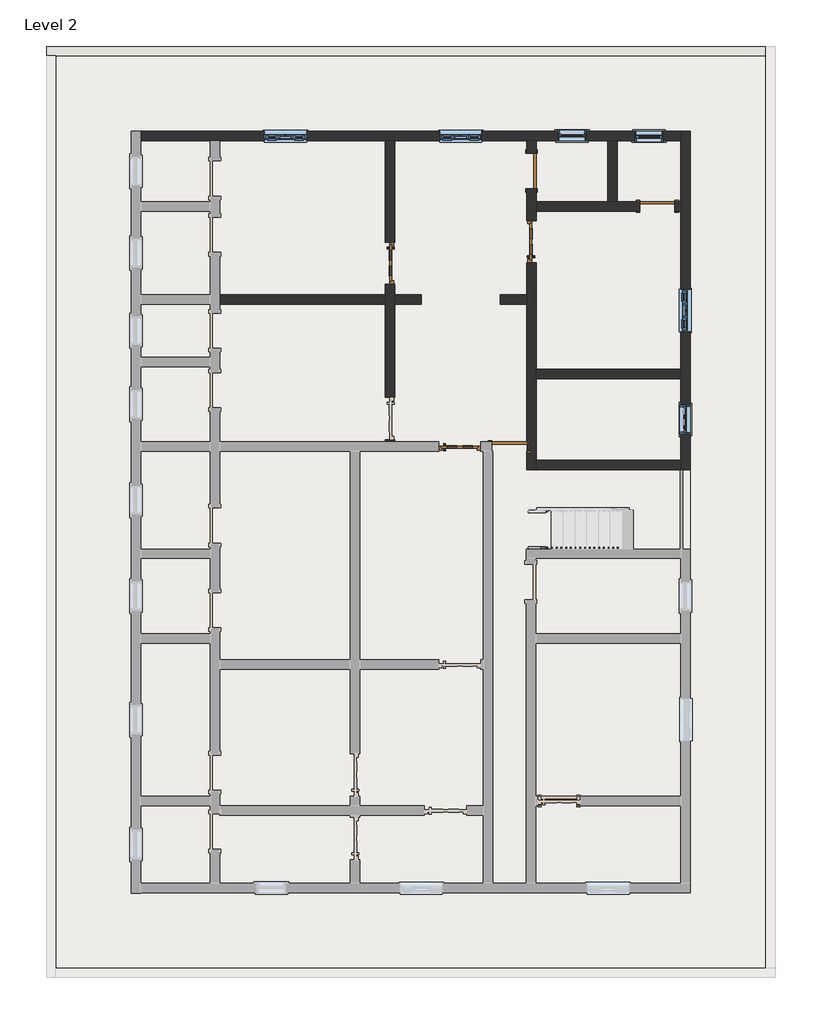
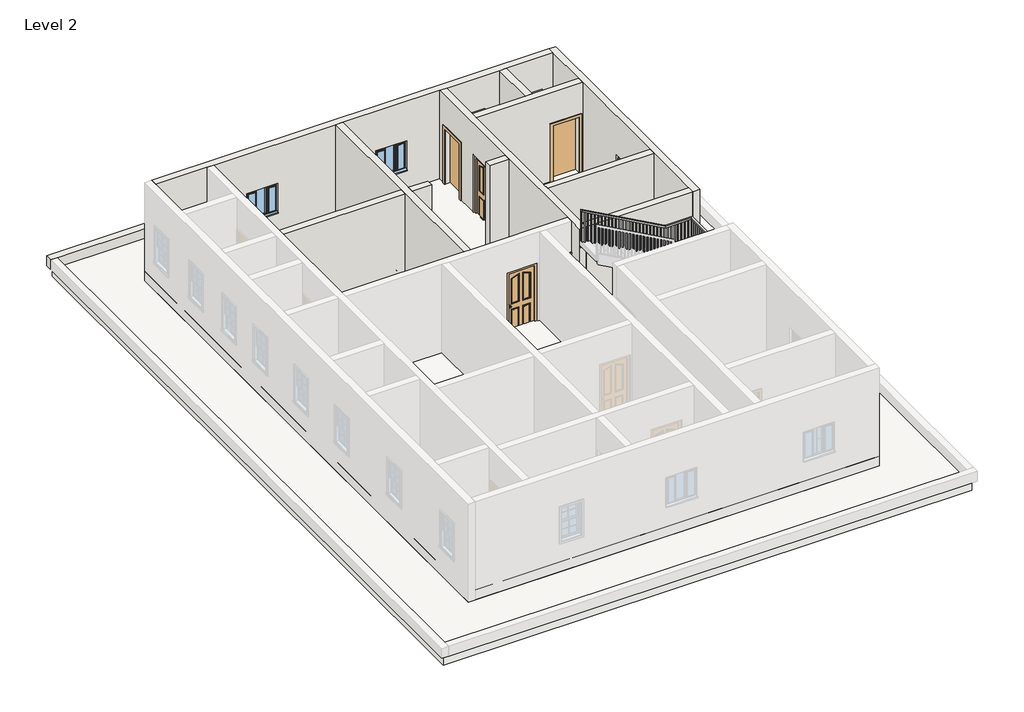
# One storey, part 2 of 3: 11 walls, 6 doors, 6 windows, 2 slabs, 1 railing, 1 roof.
# Revit data of these elements (continued)
# Type "Windows_Tpl_w-Glazing_Cross-Bars : 910x910mm" (continued)
#   Cavity Closer Depth = 0' - 3.34646"
#   Vis - Glazing Bars = yes
#   Vis - Cavity Closers = yes
#   Define Thermal Properties by = 1
#   Material Trim = Window Frame
#   Material Glazing Bars = Window Frame
#   Material Glass = Glass
#   Material Frame = Window Frame
#   Wall Closure = (empty or 0)
# Elements 1, 2, 3 (IfcDoor, "Doors_ExtSgl_12 : 910x2110mm")
#   Phase Created = New Construction
#   Materials on its faces: "Door - Panel", "Door - Handle", "Door - Frame/Mullion", "Door - Glazing"
# Elements 4, 5, 6 (IfcDoor, "Single-Flush : 30\" x 80\"")
#   Phase Created = New Construction
#   Materials on its faces: "Door - Frame", "Door - Panel"
# Element 7 (IfcRailing, "Handrail - Rectangular")
#   Phase Created = New Construction
# Element 8 (IfcRoof, "Generic - 12\"")
#   built-in parameter 1001705 = 11 (stored number, unit not read)
#   built-in parameter 1001710 = 33615
#   Phase Created = New Construction
#   Materials on its faces: "Default Roof"
# Elements 9, 10 (IfcSlab, "Generic - 12\"")
#   Height Offset From Level = 0' - 0"
#   Phase Created = New Construction
#   Materials on its faces: "Default Floor"
# Elements 11, 12, 13, 14, 15, 17, 18 (IfcWall, "4.5\"")
#   Top Offset = 0' - 0"
#   Base Offset = 0' - 0"
#   wall height = 10' - 0"
#   Phase Created = New Construction
#   Base Constraint = Level 2
#   Top Constraint = Level 3
#   Materials on its faces: "Default Wall"
# Element 16 (IfcWall, "4.5\"")
#   Top Offset = 0' - 0"
#   Base Offset = 0' - 0"
#   wall height = 10' - 0"
#   Phase Created = New Construction
#   Base Constraint = Level 2
#   Top Constraint = Level 3
#   Materials on its faces: "Default Wall", "Tile, Porcelain, 4in"
# Element 19 (IfcWall, "4.5\"")
#   Top Offset = 0' - 0"
#   Base Offset = 0' - 0"
#   Unconnected Height = 1' - 0"
#   wall height = 1' - 0"
#   Phase Created = New Construction
#   Base Constraint = Level 2
#   Materials on its faces: "Default Wall"
# Elements 20, 21 (IfcWall, "Generic - 9\"")
#   Top Offset = 0' - 0"
#   Base Offset = 0' - 0"
#   wall height = 10' - 0"
#   Phase Created = New Construction
#   Base Constraint = Level 2
#   Top Constraint = Level 3
#   Materials on its faces: "Default Wall", "Tile, Porcelain, 4in"
# Element 22 (IfcWindow, "Window-Double-Hung : 24\" x 42\"")
#   Mark = "33"
#   Window Inset = 0' - 0"
#   Interior Wall Closure = 0' - 1 1/2"
#   Frame Extension = 0' - 1 1/4"
#   Exterior Wall Closure = 0' - 0 1/2"
#   Interior Trim Visibility = yes
#   Indicator Visibility = yes
#   Exterior Trim Visibility = yes
#   Phase Created = New Construction
#   Materials on its faces: "Wood - Stained", "Glass", "Clad - White"
# Element 23 (IfcWindow, "Window-Double-Hung : 24\" x 42\"")
#   Mark = "34"
#   Window Inset = 0' - 0"
#   Interior Wall Closure = 0' - 1 1/2"
#   Frame Extension = 0' - 1 1/4"
#   Exterior Wall Closure = 0' - 0 1/2"
#   Interior Trim Visibility = yes
#   Indicator Visibility = yes
#   Exterior Trim Visibility = yes
#   Phase Created = New Construction
#   Materials on its faces: "Wood - Stained", "Glass", "Clad - White"
# Element 24 (IfcWindow, "Window-Double-Hung : 24\" x 42\"")
#   Mark = "35"
#   Window Inset = 0' - 0"
#   Interior Wall Closure = 0' - 1 1/2"
#   Frame Extension = 0' - 1 1/4"
#   Exterior Wall Closure = 0' - 0 1/2"
#   Interior Trim Visibility = yes
#   Indicator Visibility = yes
#   Exterior Trim Visibility = yes
#   Phase Created = New Construction
#   Materials on its faces: "Wood - Stained", "Glass", "Clad - White"
# Element 25 (IfcWindow, "Windows_Tpl_w-Glazing_Cross-Bars : 910x910mm")
#   Mark = "21"
#   Phase Created = New Construction
#   Materials on its faces: "Window Frame", "Glass"
# Element 26 (IfcWindow, "Windows_Tpl_w-Glazing_Cross-Bars : 910x910mm")
#   Mark = "22"
#   Phase Created = New Construction
#   Materials on its faces: "Window Frame", "Glass"
# Element 27 (IfcWindow, "Windows_Tpl_w-Glazing_Cross-Bars : 910x910mm")
#   Mark = "36"
#   Phase Created = New Construction
#   Materials on its faces: "Window Frame", "Glass"
# Materials
#   "Door - Glazing": colour RGB 0 0 255, transparency 0.75
#   "Door - Panel": class "Wood", colour RGB 210 159 95, transparency 0, Cost = 0
#   "Door - Frame/Mullion": class "Wood", colour RGB 212 179 113, transparency 0
#   "Door - Handle": colour RGB 246 240 166, transparency 0
#   "Door - Frame": colour RGB 118 70 51, transparency 0, Cost = 0
#   "Wood - Stained": class "Wood", colour RGB 224 178 126, transparency 0, Cost = 0
#   "Clad - White": class "Wood", colour RGB 242 242 238, transparency 0, Cost = 0
#   "Glass": class "Glass", colour RGB 0 128 192, transparency 0.75, Description = "Soda Lime Glass", Cost = 0
#   "Window Frame": colour RGB 249 249 249, transparency 0
#   "Default Roof": colour RGB 88 101 114, transparency 0, Cost = 0
#   "Default Floor": colour RGB 128 128 128, transparency 0, Cost = 0
#   "Default Wall": colour RGB 128 128 128, transparency 0, Cost = 0
#   "Tile, Porcelain, 4in": class "Generic", colour RGB 89 87 158, transparency 0, Description = "Porcelain tile, 4\", white", Cost = 0
